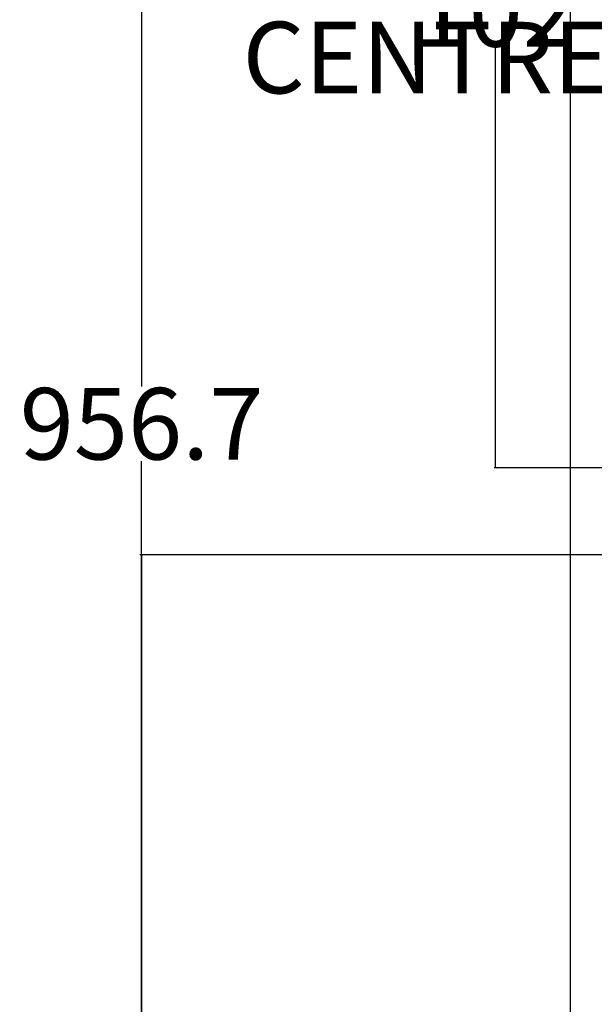
# Model space of a CAD drawing. Units: inches. Extents: x -48 to 50072, y 0 to 21068.
# Tile 46 of 75: x -48 to 16, y 628 to 738. Entities that reach past the tile are written whole.
import ezdxf

# ---------------------------------------------------------------- set-up
doc = ezdxf.new("R2010")
doc.units = ezdxf.units.IN
doc.header["$MEASUREMENT"] = 0
doc.layers.add('A-ANNO-DIMS', color=2, linetype='Continuous', lineweight=18)
doc.layers.add('C-PROP', color=7, linetype='Continuous', lineweight=25)
doc.styles.get("Standard").update_dxf_attribs({"font": 'arial.ttf'})
doc.dimstyles.get("Standard").update_dxf_attribs({"dimtxt": 8, "dimasz": 0.18, "dimexe": 0.18, "dimexo": 0.0625, "dimgap": 0.09, "dimtad": 0, "dimtih": 1, "dimtoh": 1, "dimdec": 1, "dimzin": 0, "dimdsep": 46, "dimlunit": 4, "dimtxsty": 'Standard', "dimblk": 'ARCHTICK', "dimcen": 0.09, "dimadec": 0, "dimazin": 0, "dimtfac": 1, "dimtdec": 1, "dimtofl": 0, "dimtmove": 0, "dimatfit": 3, "dimldrblk": 'ARCHTICK', "dimfxl": 1, "dimtolj": 1, "dimtzin": 0, "dimarcsym": 0})

# ---------------------------------------------------------------- blocks, each defined once
blk = doc.blocks.new('_ArchTick')
at = {"color": 0, "linetype": 'ByBlock', "const_width": 0.15}
blk.add_lwpolyline([(-0.5, -0.5), (0.5, 0.5)], dxfattribs=at)
blk = doc.blocks.new('*D106')
at = {"layer": 'A-ANNO-DIMS', "color": 0, "lineweight": -2, "transparency": 16777216}
for p, q in [((72.04, 738.93), (72.04, 733.18)), ((109.54, 738.93), (109.54, 733.18)), ((72.04, 733.36), (71.86, 733.36)), ((109.54, 733.36), (72.04, 733.36))]:
    blk.add_line(p, q, dxfattribs=at)
at = {"layer": 'Defpoints', "color": 0, "transparency": 16777216}
for p in [(72.04, 738.99), (109.54, 738.99), (72.04, 733.36)]:
    blk.add_point(p, dxfattribs=at)
at = {"layer": 'A-ANNO-DIMS', "color": 0, "lineweight": -2, "transparency": 16777216, "xscale": 0.18, "yscale": 0.18, "zscale": 0.18, "rotation": 180}
blk.add_blockref('_ArchTick', (72.04, 733.36), dxfattribs=at)
at = {"layer": 'A-ANNO-DIMS', "color": 0, "lineweight": -2, "transparency": 16777216, "xscale": 0.18, "yscale": 0.18, "zscale": 0.18}
blk.add_blockref('_ArchTick', (109.54, 733.36), dxfattribs=at)
at = {"layer": 'A-ANNO-DIMS', "color": 0, "transparency": 16777216, "insert": (22.3, 733.36), "char_height": 8, "attachment_point": 5}
blk.add_mtext('\\A1;CENTRE TABLE 38', dxfattribs=at)
blk = doc.blocks.new('*D109')
at = {"layer": 'A-ANNO-DIMS', "color": 0, "lineweight": -2, "transparency": 16777216}
for p, q in [((24.03, 789.68), (4.99, 789.68)), ((5.17, 789.68), (5.17, 742.76)), ((5.17, 687.48), (5.17, 734.41)), ((24.03, 687.48), (4.99, 687.48))]:
    blk.add_line(p, q, dxfattribs=at)
at = {"layer": 'Defpoints', "color": 0, "transparency": 16777216}
for p in [(5.17, 789.68), (24.1, 789.68), (24.1, 687.48)]:
    blk.add_point(p, dxfattribs=at)
at = {"layer": 'A-ANNO-DIMS', "color": 0, "lineweight": -2, "transparency": 16777216, "xscale": 0.18, "yscale": 0.18, "zscale": 0.18}
for p, rotation in [((5.17, 789.68), 90), ((5.17, 687.48), 270)]:
    blk.add_blockref('_ArchTick', p, dxfattribs=dict(at, rotation=rotation))
at = {"layer": 'A-ANNO-DIMS', "color": 0, "transparency": 16777216, "insert": (5.17, 738.58), "char_height": 8, "attachment_point": 5}
blk.add_mtext('\\A1;102', dxfattribs=at)
blk = doc.blocks.new('*D113')
at = {"layer": 'A-ANNO-DIMS', "color": 0, "lineweight": -2, "transparency": 16777216}
for p, q in [((13.45, 1170.77), (-34.61, 1170.77)), ((-34.43, 1170.77), (-34.43, 696.6)), ((-34.43, 214.07), (-34.43, 688.25)), ((13.45, 214.07), (-34.61, 214.07))]:
    blk.add_line(p, q, dxfattribs=at)
at = {"layer": 'Defpoints', "color": 0, "transparency": 16777216}
for p in [(-34.43, 1170.77), (13.52, 1170.77), (13.52, 214.07)]:
    blk.add_point(p, dxfattribs=at)
at = {"layer": 'A-ANNO-DIMS', "color": 0, "lineweight": -2, "transparency": 16777216, "xscale": 0.18, "yscale": 0.18, "zscale": 0.18}
for p, rotation in [((-34.43, 1170.77), 90), ((-34.43, 214.07), 270)]:
    blk.add_blockref('_ArchTick', p, dxfattribs=dict(at, rotation=rotation))
at = {"layer": 'A-ANNO-DIMS', "color": 0, "transparency": 16777216, "insert": (-34.43, 692.42), "char_height": 8, "attachment_point": 5}
blk.add_mtext('\\A1;956.7', dxfattribs=at)
blk = doc.blocks.new('*D127')
at = {"layer": 'A-ANNO-DIMS', "color": 0, "lineweight": -2, "transparency": 16777216}
for p, q in [((215.95, 677.77), (-34.61, 677.77)), ((-34.43, 677.77), (-34.43, 587.45)), ((-34.43, 488.77), (-34.43, 579.1)), ((215.95, 488.77), (-34.61, 488.77))]:
    blk.add_line(p, q, dxfattribs=at)
at = {"layer": 'Defpoints', "color": 0, "transparency": 16777216}
for p in [(-34.43, 677.77), (216.02, 677.77), (216.02, 488.77)]:
    blk.add_point(p, dxfattribs=at)
at = {"layer": 'A-ANNO-DIMS', "color": 0, "lineweight": -2, "transparency": 16777216, "xscale": 0.18, "yscale": 0.18, "zscale": 0.18}
for p, rotation in [((-34.43, 677.77), 90), ((-34.43, 488.77), 270)]:
    blk.add_blockref('_ArchTick', p, dxfattribs=dict(at, rotation=rotation))
at = {"layer": 'A-ANNO-DIMS', "color": 0, "transparency": 16777216, "insert": (-34.43, 583.27), "char_height": 8, "attachment_point": 5}
blk.add_mtext('\\A1;189', dxfattribs=at)

msp = doc.modelspace()

# ---------------------------------------------------------------- linework, layer by layer
at = {"layer": 'C-PROP'}
msp.add_line((13.517, 1170.775), (13.517, 214.075), dxfattribs=at)

# ---------------------------------------------------------------- dimensions: what is measured, and where the dimension line sits
at = {"layer": 'A-ANNO-DIMS'}
for base, p1, p2, override, picture, middle in [((-34.433, 1170.775), (13.517, 214.075), (13.517, 1170.775), {"dimdec": 1, "dimlfac": 1, "dimrnd": 0, "dimzin": 0, "dimdsep": 46, "dimlunit": 2}, '*D113', (-34.433, 692.425)), ((5.167, 789.685), (24.097, 687.484), (24.097, 789.685), {"dimdec": 0, "dimlfac": 1, "dimrnd": 0, "dimzin": 0, "dimdsep": 46, "dimlunit": 2}, '*D109', (5.167, 738.584)), ((-34.433, 677.775), (216.017, 488.775), (216.017, 677.775), {"dimdec": 0, "dimlfac": 1, "dimrnd": 0, "dimzin": 0, "dimdsep": 46, "dimlunit": 2}, '*D127', (-34.433, 583.275))]:
    dim = msp.add_linear_dim(base=base, p1=p1, p2=p2, angle=90, dimstyle='Standard', override=override, dxfattribs=at)
    dim.commit()
    dim.dimension.update_dxf_attribs({"geometry": picture, "text_midpoint": middle})
dim = msp.add_linear_dim(base=(72.042451158, 733.362887343), p1=(109.542451158, 738.987887343), p2=(72.042451158, 738.987887343), angle=180, text='CENTRE TABLE <>', dimstyle='Standard', override={"dimdec": 0, "dimlfac": 1, "dimrnd": 0, "dimzin": 0, "dimdsep": 46, "dimlunit": 2}, dxfattribs=at)
dim.commit()
dim.dimension.update_dxf_attribs({"geometry": '*D106', "text_midpoint": (22.29905416, 733.362887343)})

doc.saveas('drawing.dxf')
